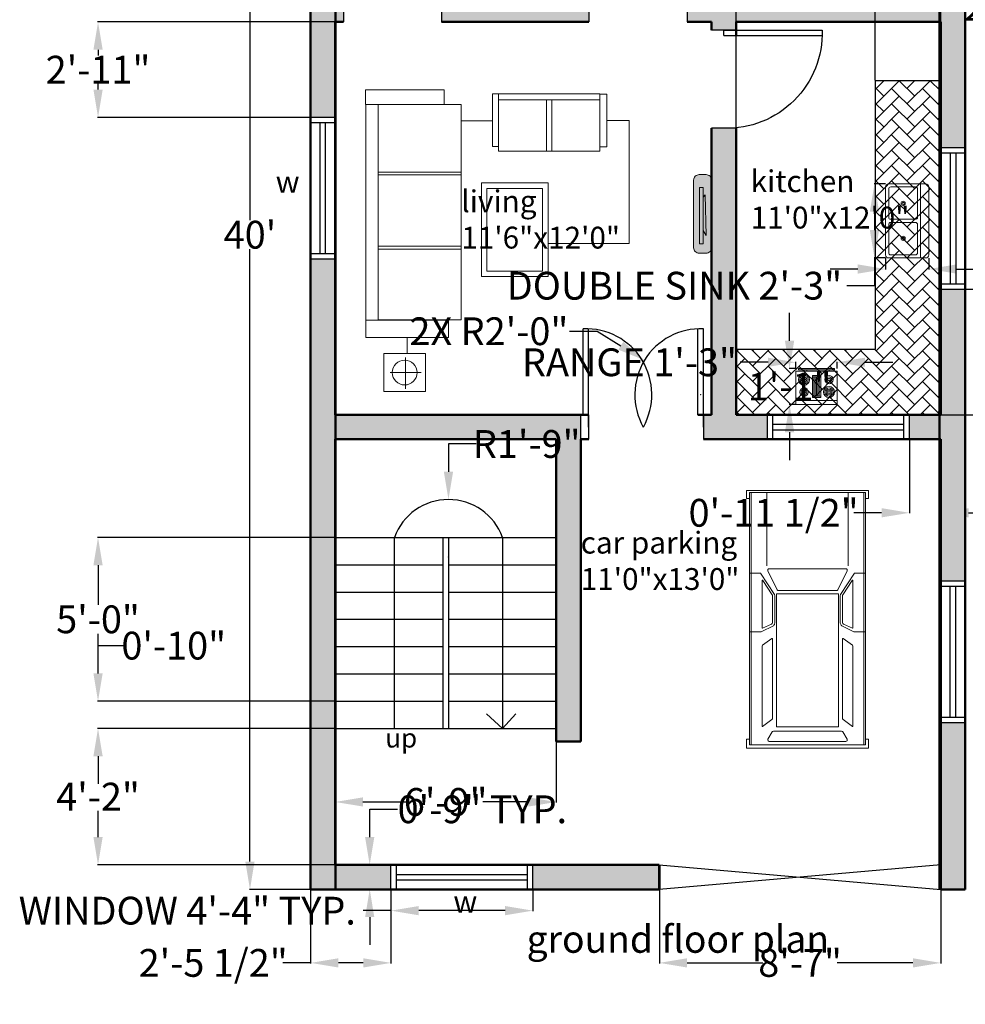
# Model space of a CAD drawing. Units: inches. Extents: x 4451 to 5261, y 886 to 1442.
# Tile 1 of 4: x 4460 to 4807, y 886 to 1247. Entities that reach past the tile are written whole.
import ezdxf

# ---------------------------------------------------------------- set-up
doc = ezdxf.new("R2010")
doc.units = ezdxf.units.IN
doc.header["$MEASUREMENT"] = 0
for name, color, linetype, lineweight in [('A-ANNO-DIMS', 2, 'Continuous', 18), ('A-ANNO-TEXT', 7, 'Continuous', 25), ('A-AREA-IDEN', 7, 'Continuous', 25), ('A-CASE', 9, 'Continuous', 25), ('A-DOOR', 4, 'Continuous', 25), ('A-FLOR-FIXT', 9, 'Continuous', 20), ('A-FLOR-STRS', 7, 'Continuous', 25), ('A-FURN', 8, 'Continuous', 18), ('A-FURN-PATT', 8, 'Continuous', 13), ('A-GLAZ', 4, 'Continuous', 25), ('A-SITE-VEHI', 8, 'Continuous', 13), ('A-WALL', 7, 'Continuous', 50), ('A-WALL-PATT', 252, 'Continuous', 13)]:
    doc.layers.add(name, color=color, linetype=linetype, lineweight=lineweight)
doc.layers.add('A-CASE-PATT', color=11, linetype='Continuous', lineweight=13, true_color=0xf27172)
doc.layers.add('A-EQPM', color=241, linetype='Continuous', lineweight=18, true_color=0xf7abae)
doc.styles.get("Standard").update_dxf_attribs({"font": 'arial.ttf'})
doc.dimstyles.get("Standard").update_dxf_attribs({"dimtxt": 10.18, "dimasz": 10.18, "dimexe": 0.18, "dimexo": 0.0625, "dimgap": 0.09, "dimtad": 0, "dimtih": 1, "dimtoh": 1, "dimdec": 0, "dimzin": 0, "dimdsep": 46, "dimlunit": 3, "dimtxsty": 'Standard', "dimcen": 0.09, "dimadec": 0, "dimazin": 0, "dimtfac": 1, "dimtdec": 0, "dimtofl": 0, "dimtmove": 0, "dimatfit": 3, "dimfxl": 1, "dimtolj": 1, "dimtzin": 0, "dimarcsym": 0})

# ---------------------------------------------------------------- blocks, each defined once
blk = doc.blocks.new('*U5')
for p, q in [((1.28, 38.87), (175.66, 38.87)), ((1.28, 28.15), (52.13, 28.15)), ((1.28, -28.15), (52.13, -28.15)), ((1.28, -38.87), (175.66, -38.87))]:
    blk.add_line(p, q)
for points in [[(5.57, 40.01), (5.57, 42.18), (0, 42.18), (0, -42.18), (5.57, -42.18), (5.57, -40.01), (1.28, -40.01), (1.28, 40.01)], [(171.74, 40.01), (175.66, 40.01), (175.66, -40.01), (171.74, -40.01), (171.74, -42.18), (178.14, -42.18), (178.14, 42.18), (171.74, 42.18)], [(1.28, 40.01), (175.66, 40.01), (175.66, -40.01), (1.28, -40.01)], [(71.47, 21.48), (163.42, 21.48), (163.42, -21.48), (71.47, -21.48)]]:
    blk.add_lwpolyline(points, close=True)
for points in [[(57.15, 40.01), (57.15, 32.39), (71.72, 22.83, 0.086577), (72.56, 22.68), (91.59, 22.68, 0.227875), (93.54, 23.62), (97.72, 32.11), (97.72, 40.01)], [(57.15, -40.01), (57.15, -32.39), (71.72, -22.83, -0.086577), (72.56, -22.68), (91.59, -22.68, -0.227875), (93.54, -23.62), (97.72, -32.11), (97.72, -40.01)]]:
    blk.add_lwpolyline(points, format="xyb")
for points in [[(55.49, 27.42), (68.59, 20.89, -0.284287), (69.14, 19.99), (69.14, -19.99, -0.284287), (68.59, -20.89), (55.49, -27.42, -0.557284), (54.05, -26.53), (54.05, 26.53, -0.557284)], [(62.08, 30.95), (72.14, 24.35, 0.146139), (72.69, 24.18), (91.42, 24.18, 0.29766), (92.33, 24.78), (95.09, 31.05, 0.541236), (94.86, 31.41), (62.21, 31.41, 0.744989)], [(102.19, 24.58), (106.97, 31, -0.236929), (107.78, 31.41), (162.91, 31.41, -0.621576), (163.11, 31), (158.19, 24.58, -0.233368), (157.39, 24.18), (102.39, 24.18, -0.616908)], [(171.88, 27.31), (166.83, 24.47, 0.271143), (166.32, 23.6), (166.32, -23.6, 0.271143), (166.83, -24.47), (171.88, -27.31, 0.573387), (173.37, -26.44), (173.37, 26.44, 0.573387)], [(62.08, -30.95), (72.14, -24.35, -0.146139), (72.69, -24.18), (91.42, -24.18, -0.29766), (92.33, -24.78), (95.09, -31.05, -0.541236), (94.86, -31.41), (62.21, -31.41, -0.744989)], [(102.19, -24.58), (106.97, -31, 0.236929), (107.78, -31.41), (162.91, -31.41, 0.621576), (163.11, -31), (158.19, -24.58, 0.233368), (157.39, -24.18), (102.39, -24.18, 0.616908)]]:
    blk.add_lwpolyline(points, format="xyb", close=True)
blk = doc.blocks.new('Range-Oven - 30 in top')
for p, q in [((0, -3), (30, -3)), ((12, -6), (18, -6)), ((13, -20), (13, -6)), ((14, -6), (14, -20)), ((15, -20), (15, -6)), ((16, -6), (16, -20)), ((17, -20), (17, -6)), ((18, -20), (12, -20)), ((6, -24), (6, -25)), ((8, -25), (8, -24)), ((22, -25), (22, -24)), ((24, -24), (24, -25))]:
    blk.add_line(p, q)
for points in [[(0, -24), (0, 0), (30, 0), (30, -24)], [(12, -21), (12, -5), (18, -5), (18, -21)], [(2, -26), (2, -25), (28, -25), (28, -26)]]:
    blk.add_lwpolyline(points, close=True)
for centre, radius in [((6, -9), 4), ((6, -9), 3), ((6, -9), 2), ((24, -9), 3), ((24, -9), 2), ((6, -9), 1), ((24, -18), 4), ((24, -9), 1), ((6, -18), 3), ((6, -18), 2), ((6, -18), 1), ((24, -18), 3), ((24, -18), 2), ((24, -18), 1)]:
    blk.add_circle(centre, radius)
blk = doc.blocks.new('Sink-double - 36 in top')
for p, q in [((-18, -4), (18, -4)), ((-0.75, -18.5), (-0.75, -6.5)), ((0.75, -6.5), (0.75, -18.5))]:
    blk.add_line(p, q)
for points in [[(-16.5, 0), (16.5, 0)], [(-18, -19.5), (-18, -1.5)], [(18, -1.5), (18, -19.5)], [(-16.5, -18.5), (-16.5, -6.5)], [(-15.5, -5.5), (-1.75, -5.5)], [(1.75, -5.5), (15.5, -5.5)], [(16.5, -6.5), (16.5, -18.5)], [(16.5, -21), (-16.5, -21)], [(-1.75, -19.5), (-15.5, -19.5)], [(15.5, -19.5), (1.75, -19.5)]]:
    blk.add_lwpolyline(points)
for centre, radius in [((-8.5, -12.5), 1), ((-8.5, -12.5), 0.5), ((8.5, -12.5), 1), ((8.5, -12.5), 0.5)]:
    blk.add_circle(centre, radius)
for centre, radius, start, end in [((-16.5, -1.5), 1.5, 90, 180), ((16.5, -1.5), 1.5, 0, 90), ((-15.5, -6.5), 1, 90, 180), ((-1.75, -6.5), 1, 0, 90), ((1.75, -6.5), 1, 90, 180), ((15.5, -6.5), 1, 0, 90), ((-15.5, -18.5), 1, 180, 270), ((-1.75, -18.5), 1, 270, 0), ((1.75, -18.5), 1, 180, 270), ((15.5, -18.5), 1, 270, 0), ((-16.5, -19.5), 1.5, 180, 270), ((16.5, -19.5), 1.5, 270, 0)]:
    blk.add_arc(centre, radius, start, end)
blk = doc.blocks.new('*D12')
at = {"layer": 'A-ANNO-DIMS', "color": 0, "lineweight": -2, "transparency": 16777216}
for p, q in [((4567.03, 1408.25), (4544.66, 1408.25)), ((4544.84, 1398.07), (4544.84, 1173.54)), ((4544.84, 938.43), (4544.84, 1162.96)), ((4567.03, 928.25), (4544.66, 928.25))]:
    blk.add_line(p, q, dxfattribs=at)
at = {"layer": 'A-ANNO-DIMS', "color": 0, "transparency": 16777216}
for points in [[(4543.14, 1398.07), (4546.53, 1398.07), (4544.84, 1408.25)], [(4543.14, 938.43), (4546.53, 938.43), (4544.84, 928.25)]]:
    blk.add_solid(points, dxfattribs=at)
at = {"layer": 'Defpoints', "color": 0, "transparency": 16777216}
for p in [(4567.09, 1408.25), (4544.84, 928.25), (4567.09, 928.25)]:
    blk.add_point(p, dxfattribs=at)
at = {"layer": 'A-ANNO-DIMS', "color": 0, "transparency": 16777216, "insert": (4544.84, 1168.25), "char_height": 10.18, "attachment_point": 5}
blk.add_mtext("\\A1;40'", dxfattribs=at)
blk = doc.blocks.new('DOOR-36-SWING')
for p, q in [((36.01, 36.01), (0.01, 36.01)), ((36.01, 34.01), (0.01, 34.01)), ((31.51, 36.01), (40.51, 36.01)), ((36.01, 34.01), (36.01, 36.01)), ((31.51, 0.01), (40.51, 0.01))]:
    blk.add_line(p, q)
blk.add_arc((35.01, 35.01), 35.01, 178.3634, 271.6366)
blk = doc.blocks.new('WIN-48-PLAN')
for p, q in [((0, 52), (9, 52)), ((0, 50), (9, 50)), ((3.5, 50), (3.5, 2)), ((5.5, 50), (5.5, 2)), ((0, 2), (9, 2)), ((0, 0), (9, 0))]:
    blk.add_line(p, q)
blk = doc.blocks.new('*D21')
at = {"layer": 'A-ANNO-DIMS', "color": 0, "lineweight": -2, "transparency": 16777216}
for p, q in [((4596.54, 928.19), (4596.54, 920.27)), ((4648.54, 928.19), (4648.54, 920.27)), ((4596.54, 920.45), (4586.36, 920.45)), ((4638.36, 920.45), (4606.72, 920.45))]:
    blk.add_line(p, q, dxfattribs=at)
at = {"layer": 'A-ANNO-DIMS', "color": 0, "transparency": 16777216}
for points in [[(4606.72, 922.15), (4606.72, 918.76), (4596.54, 920.45)], [(4638.36, 922.15), (4638.36, 918.76), (4648.54, 920.45)]]:
    blk.add_solid(points, dxfattribs=at)
at = {"layer": 'Defpoints', "color": 0, "transparency": 16777216}
for p in [(4596.54, 928.25), (4648.54, 928.25), (4596.54, 920.45)]:
    blk.add_point(p, dxfattribs=at)
at = {"layer": 'A-ANNO-DIMS', "color": 0, "transparency": 16777216, "insert": (4521.86, 920.45), "char_height": 10.18, "attachment_point": 5}
blk.add_mtext('\\A1;WINDOW 4\'-4" TYP.', dxfattribs=at)
blk = doc.blocks.new('*D22')
at = {"layer": 'A-ANNO-DIMS', "color": 0, "lineweight": -2, "transparency": 16777216}
for p, q in [((4588.74, 947.43), (4588.74, 957.61)), ((4588.74, 957.61), (4598.92, 957.61)), ((4596.47, 937.25), (4588.56, 937.25)), ((4596.47, 928.25), (4588.56, 928.25)), ((4588.74, 918.07), (4588.74, 907.89))]:
    blk.add_line(p, q, dxfattribs=at)
at = {"layer": 'A-ANNO-DIMS', "color": 0, "transparency": 16777216}
for points in [[(4587.04, 947.43), (4590.43, 947.43), (4588.74, 937.25)], [(4587.04, 918.07), (4590.43, 918.07), (4588.74, 928.25)]]:
    blk.add_solid(points, dxfattribs=at)
at = {"layer": 'Defpoints', "color": 0, "transparency": 16777216}
for p in [(4588.74, 937.25), (4596.54, 937.25), (4596.54, 928.25)]:
    blk.add_point(p, dxfattribs=at)
at = {"layer": 'A-ANNO-DIMS', "color": 0, "transparency": 16777216, "insert": (4630.03, 957.61), "char_height": 10.18, "attachment_point": 5}
blk.add_mtext('\\A1;0\'-9" TYP.', dxfattribs=at)
blk = doc.blocks.new('*D27')
at = {"layer": 'A-ANNO-DIMS', "color": 0, "lineweight": -2, "transparency": 16777216}
for p, q in [((4734.76, 1121.48), (4724.58, 1121.48)), ((4744.94, 1119.26), (4744.94, 1121.66)), ((4760.17, 1119.26), (4760.17, 1121.66)), ((4770.35, 1121.48), (4780.53, 1121.48))]:
    blk.add_line(p, q, dxfattribs=at)
at = {"layer": 'A-ANNO-DIMS', "color": 0, "transparency": 16777216}
for points in [[(4734.76, 1123.18), (4734.76, 1119.79), (4744.94, 1121.48)], [(4770.35, 1123.18), (4770.35, 1119.79), (4760.17, 1121.48)]]:
    blk.add_solid(points, dxfattribs=at)
at = {"layer": 'Defpoints', "color": 0, "transparency": 16777216}
for p in [(4744.94, 1121.48), (4744.94, 1119.2), (4760.17, 1119.2)]:
    blk.add_point(p, dxfattribs=at)
at = {"layer": 'A-ANNO-DIMS', "color": 0, "transparency": 16777216, "insert": (4683.96, 1121.48), "char_height": 10.18, "attachment_point": 5}
blk.add_mtext('\\A1;RANGE 1\'-3"', dxfattribs=at)
blk = doc.blocks.new('*D28')
at = {"layer": 'A-ANNO-DIMS', "color": 0, "lineweight": -2, "transparency": 16777216}
for p, q in [((4742.66, 1129.38), (4742.66, 1139.56)), ((4744.88, 1119.2), (4742.48, 1119.2)), ((4744.88, 1106), (4742.48, 1106)), ((4742.66, 1095.82), (4742.66, 1085.64))]:
    blk.add_line(p, q, dxfattribs=at)
at = {"layer": 'A-ANNO-DIMS', "color": 0, "transparency": 16777216}
for points in [[(4740.96, 1129.38), (4744.36, 1129.38), (4742.66, 1119.2)], [(4740.96, 1095.82), (4744.36, 1095.82), (4742.66, 1106)]]:
    blk.add_solid(points, dxfattribs=at)
at = {"layer": 'Defpoints', "color": 0, "transparency": 16777216}
for p in [(4744.94, 1119.2), (4742.66, 1106), (4744.94, 1106)]:
    blk.add_point(p, dxfattribs=at)
at = {"layer": 'A-ANNO-DIMS', "color": 0, "transparency": 16777216, "insert": (4742.66, 1112.6), "char_height": 10.18, "attachment_point": 5}
blk.add_mtext('\\A1;1\'-1"', dxfattribs=at)
blk = doc.blocks.new('*D29')
at = {"layer": 'A-ANNO-DIMS', "color": 0, "lineweight": -2, "transparency": 16777216}
for p, q in [((4777.81, 1186.9), (4773.62, 1186.9)), ((4773.8, 1176.72), (4773.8, 1169.92)), ((4777.81, 1159.74), (4773.62, 1159.74)), ((4773.8, 1159.74), (4773.8, 1149.56)), ((4773.8, 1149.56), (4763.62, 1149.56))]:
    blk.add_line(p, q, dxfattribs=at)
at = {"layer": 'A-ANNO-DIMS', "color": 0, "transparency": 16777216}
for points in [[(4772.1, 1176.72), (4775.49, 1176.72), (4773.8, 1186.9)], [(4772.1, 1169.92), (4775.49, 1169.92), (4773.8, 1159.74)]]:
    blk.add_solid(points, dxfattribs=at)
at = {"layer": 'Defpoints', "color": 0, "transparency": 16777216}
for p in [(4777.87, 1186.9), (4773.8, 1159.74), (4777.87, 1159.74)]:
    blk.add_point(p, dxfattribs=at)
at = {"layer": 'A-ANNO-DIMS', "color": 0, "transparency": 16777216, "insert": (4700.46, 1149.56), "char_height": 10.18, "attachment_point": 5}
blk.add_mtext('\\A1;DOUBLE SINK 2\'-3"', dxfattribs=at)
blk = doc.blocks.new('*D30')
at = {"layer": 'A-ANNO-DIMS', "color": 0, "lineweight": -2, "transparency": 16777216}
for p, q in [((4777.87, 1159.67), (4777.87, 1155.48)), ((4793.72, 1159.67), (4793.72, 1155.48)), ((4767.69, 1155.66), (4757.51, 1155.66)), ((4803.9, 1155.66), (4814.08, 1155.66))]:
    blk.add_line(p, q, dxfattribs=at)
at = {"layer": 'A-ANNO-DIMS', "color": 0, "transparency": 16777216}
for points in [[(4767.69, 1157.36), (4767.69, 1153.97), (4777.87, 1155.66)], [(4803.9, 1157.36), (4803.9, 1153.97), (4793.72, 1155.66)]]:
    blk.add_solid(points, dxfattribs=at)
at = {"layer": 'Defpoints', "color": 0, "transparency": 16777216}
for p in [(4777.87, 1159.74), (4793.72, 1159.74), (4793.72, 1155.66)]:
    blk.add_point(p, dxfattribs=at)
at = {"layer": 'A-ANNO-DIMS', "color": 0, "transparency": 16777216, "insert": (4827.22, 1155.66), "char_height": 10.18, "attachment_point": 5}
blk.add_mtext('\\A1;1\'-4"', dxfattribs=at)
blk = doc.blocks.new('*D41')
at = {"layer": 'A-ANNO-DIMS', "color": 0, "lineweight": -2, "transparency": 16777216}
for p, q in [((4723.09, 1102.31), (4723.09, 1435.38)), ((4733.27, 1435.2), (4746.94, 1435.2)), ((4787.91, 1435.2), (4774.24, 1435.2)), ((4798.09, 1102.31), (4798.09, 1435.38))]:
    blk.add_line(p, q, dxfattribs=at)
at = {"layer": 'A-ANNO-DIMS', "color": 0, "transparency": 16777216}
for points in [[(4733.27, 1436.9), (4733.27, 1433.51), (4723.09, 1435.2)], [(4787.91, 1436.9), (4787.91, 1433.51), (4798.09, 1435.2)]]:
    blk.add_solid(points, dxfattribs=at)
at = {"layer": 'Defpoints', "color": 0, "transparency": 16777216}
for p in [(4798.09, 1435.2), (4723.09, 1102.25), (4798.09, 1102.25)]:
    blk.add_point(p, dxfattribs=at)
at = {"layer": 'A-ANNO-DIMS', "color": 0, "transparency": 16777216, "insert": (4760.59, 1435.2), "char_height": 10.18, "attachment_point": 5}
blk.add_mtext('\\A1;6\'-3"', dxfattribs=at)
blk = doc.blocks.new('*D42')
at = {"layer": 'A-ANNO-DIMS', "color": 0, "lineweight": -2, "transparency": 16777216}
for p, q in [((4694.94, 928.2), (4694.94, 901.12)), ((4798.09, 928.19), (4798.09, 901.12)), ((4705.12, 901.3), (4732.89, 901.3)), ((4787.91, 901.3), (4760.15, 901.3))]:
    blk.add_line(p, q, dxfattribs=at)
at = {"layer": 'A-ANNO-DIMS', "color": 0, "transparency": 16777216}
for points in [[(4705.12, 903), (4705.12, 899.61), (4694.94, 901.3)], [(4787.91, 903), (4787.91, 899.61), (4798.09, 901.3)]]:
    blk.add_solid(points, dxfattribs=at)
at = {"layer": 'Defpoints', "color": 0, "transparency": 16777216}
for p in [(4694.94, 928.26), (4798.09, 928.25), (4798.09, 901.3)]:
    blk.add_point(p, dxfattribs=at)
at = {"layer": 'A-ANNO-DIMS', "color": 0, "transparency": 16777216, "insert": (4746.52, 901.3), "char_height": 10.18, "attachment_point": 5}
blk.add_mtext('\\A1;8\'-7"', dxfattribs=at)
blk = doc.blocks.new('*D43')
at = {"layer": 'A-ANNO-DIMS', "color": 0, "lineweight": -2, "transparency": 16777216}
for p, q in [((4567.09, 928.19), (4567.09, 901.12)), ((4596.54, 928.19), (4596.54, 901.12)), ((4567.09, 901.3), (4556.91, 901.3)), ((4586.36, 901.3), (4577.27, 901.3))]:
    blk.add_line(p, q, dxfattribs=at)
at = {"layer": 'A-ANNO-DIMS', "color": 0, "transparency": 16777216}
for points in [[(4577.27, 903), (4577.27, 899.61), (4567.09, 901.3)], [(4586.36, 903), (4586.36, 899.61), (4596.54, 901.3)]]:
    blk.add_solid(points, dxfattribs=at)
at = {"layer": 'Defpoints', "color": 0, "transparency": 16777216}
for p in [(4567.09, 928.25), (4596.54, 928.25), (4567.09, 901.3)]:
    blk.add_point(p, dxfattribs=at)
at = {"layer": 'A-ANNO-DIMS', "color": 0, "transparency": 16777216, "insert": (4531.35, 901.3), "char_height": 10.18, "attachment_point": 5}
blk.add_mtext('\\A1;2\'-5 1/2"', dxfattribs=at)
blk = doc.blocks.new('*D45')
at = {"layer": 'A-ANNO-DIMS', "color": 0, "lineweight": -2, "transparency": 16777216}
for p, q in [((4798.16, 1148.25), (4859.61, 1148.25)), ((4859.43, 1138.07), (4859.43, 1130.54)), ((4859.43, 1112.43), (4859.43, 1119.96)), ((4798.16, 1102.25), (4859.61, 1102.25))]:
    blk.add_line(p, q, dxfattribs=at)
at = {"layer": 'A-ANNO-DIMS', "color": 0, "transparency": 16777216}
for points in [[(4857.74, 1138.07), (4861.13, 1138.07), (4859.43, 1148.25)], [(4857.74, 1112.43), (4861.13, 1112.43), (4859.43, 1102.25)]]:
    blk.add_solid(points, dxfattribs=at)
at = {"layer": 'Defpoints', "color": 0, "transparency": 16777216}
for p in [(4798.09, 1148.25), (4859.43, 1148.25), (4798.09, 1102.25)]:
    blk.add_point(p, dxfattribs=at)
at = {"layer": 'A-ANNO-DIMS', "color": 0, "transparency": 16777216, "insert": (4859.43, 1125.25), "char_height": 10.18, "attachment_point": 5}
blk.add_mtext('\\A1;3\'-10"', dxfattribs=at)
blk = doc.blocks.new('*D48')
at = {"layer": 'A-ANNO-DIMS', "color": 0, "lineweight": -2, "transparency": 16777216}
for p, q in [((4576.03, 1246.25), (4488.96, 1246.25)), ((4489.14, 1236.07), (4489.14, 1233.95)), ((4489.14, 1221.44), (4489.14, 1223.55)), ((4576.03, 1211.26), (4488.96, 1211.26))]:
    blk.add_line(p, q, dxfattribs=at)
at = {"layer": 'A-ANNO-DIMS', "color": 0, "transparency": 16777216}
for points in [[(4487.45, 1236.07), (4490.84, 1236.07), (4489.14, 1246.25)], [(4487.45, 1221.44), (4490.84, 1221.44), (4489.14, 1211.26)]]:
    blk.add_solid(points, dxfattribs=at)
at = {"layer": 'Defpoints', "color": 0, "transparency": 16777216}
for p in [(4576.09, 1246.25), (4489.14, 1211.26), (4576.09, 1211.26)]:
    blk.add_point(p, dxfattribs=at)
at = {"layer": 'A-ANNO-DIMS', "color": 0, "transparency": 16777216, "insert": (4489.14, 1228.75), "char_height": 10.18, "attachment_point": 5}
blk.add_mtext('\\A1;2\'-11"', dxfattribs=at)
blk = doc.blocks.new('*D51')
at = {"layer": 'A-ANNO-DIMS', "color": 0, "lineweight": -2, "transparency": 16777216}
for p, q in [((4489.14, 1007.43), (4489.14, 1017.61)), ((4489.14, 1017.61), (4499.32, 1017.61)), ((4576.03, 997.25), (4488.96, 997.25)), ((4576.03, 987.25), (4488.96, 987.25)), ((4489.14, 977.07), (4489.14, 966.89))]:
    blk.add_line(p, q, dxfattribs=at)
at = {"layer": 'A-ANNO-DIMS', "color": 0, "transparency": 16777216}
for points in [[(4487.45, 1007.43), (4490.84, 1007.43), (4489.14, 997.25)], [(4487.45, 977.07), (4490.84, 977.07), (4489.14, 987.25)]]:
    blk.add_solid(points, dxfattribs=at)
at = {"layer": 'Defpoints', "color": 0, "transparency": 16777216}
for p in [(4489.14, 997.25), (4576.09, 997.25), (4576.09, 987.25)]:
    blk.add_point(p, dxfattribs=at)
at = {"layer": 'A-ANNO-DIMS', "color": 0, "transparency": 16777216, "insert": (4516.9, 1017.61), "char_height": 10.18, "attachment_point": 5}
blk.add_mtext('\\A1;0\'-10"', dxfattribs=at)
blk = doc.blocks.new('*D52')
at = {"layer": 'A-ANNO-DIMS', "color": 0, "lineweight": -2, "transparency": 16777216}
for p, q in [((4576.03, 1057.25), (4488.96, 1057.25)), ((4489.14, 1047.07), (4489.14, 1032.54)), ((4489.14, 1007.43), (4489.14, 1021.96)), ((4576.03, 997.25), (4488.96, 997.25))]:
    blk.add_line(p, q, dxfattribs=at)
at = {"layer": 'A-ANNO-DIMS', "color": 0, "transparency": 16777216}
for points in [[(4487.45, 1047.07), (4490.84, 1047.07), (4489.14, 1057.25)], [(4487.45, 1007.43), (4490.84, 1007.43), (4489.14, 997.25)]]:
    blk.add_solid(points, dxfattribs=at)
at = {"layer": 'Defpoints', "color": 0, "transparency": 16777216}
for p in [(4489.14, 1057.25), (4576.09, 1057.25), (4576.09, 997.25)]:
    blk.add_point(p, dxfattribs=at)
at = {"layer": 'A-ANNO-DIMS', "color": 0, "transparency": 16777216, "insert": (4489.14, 1027.25), "char_height": 10.18, "attachment_point": 5}
blk.add_mtext('\\A1;5\'-0"', dxfattribs=at)
blk = doc.blocks.new('*D53')
at = {"layer": 'A-ANNO-DIMS', "color": 0, "lineweight": -2, "transparency": 16777216}
for p, q in [((4576.03, 987.25), (4488.96, 987.25)), ((4489.14, 977.07), (4489.14, 967.45)), ((4489.14, 947.43), (4489.14, 957.05)), ((4576.03, 937.25), (4488.96, 937.25))]:
    blk.add_line(p, q, dxfattribs=at)
at = {"layer": 'A-ANNO-DIMS', "color": 0, "transparency": 16777216}
for points in [[(4487.45, 977.07), (4490.84, 977.07), (4489.14, 987.25)], [(4487.45, 947.43), (4490.84, 947.43), (4489.14, 937.25)]]:
    blk.add_solid(points, dxfattribs=at)
at = {"layer": 'Defpoints', "color": 0, "transparency": 16777216}
for p in [(4489.14, 987.25), (4576.09, 987.25), (4576.09, 937.25)]:
    blk.add_point(p, dxfattribs=at)
at = {"layer": 'A-ANNO-DIMS', "color": 0, "transparency": 16777216, "insert": (4489.14, 962.25), "char_height": 10.18, "attachment_point": 5}
blk.add_mtext('\\A1;4\'-2"', dxfattribs=at)
blk = doc.blocks.new('*D54')
at = {"layer": 'A-ANNO-DIMS', "color": 0, "lineweight": -2, "transparency": 16777216}
for p, q in [((4774.09, 1224.89), (4774.09, 1251.96)), ((4784.27, 1251.78), (4787.91, 1251.78)), ((4798.09, 1224.89), (4798.09, 1251.96)), ((4798.09, 1251.78), (4808.27, 1251.78))]:
    blk.add_line(p, q, dxfattribs=at)
at = {"layer": 'A-ANNO-DIMS', "color": 0, "transparency": 16777216}
for points in [[(4784.27, 1253.48), (4784.27, 1250.08), (4774.09, 1251.78)], [(4787.91, 1253.48), (4787.91, 1250.08), (4798.09, 1251.78)]]:
    blk.add_solid(points, dxfattribs=at)
at = {"layer": 'Defpoints', "color": 0, "transparency": 16777216}
for p in [(4798.09, 1251.78), (4774.09, 1224.83), (4798.09, 1224.83)]:
    blk.add_point(p, dxfattribs=at)
at = {"layer": 'A-ANNO-DIMS', "color": 0, "transparency": 16777216, "insert": (4821.98, 1251.78), "char_height": 10.18, "attachment_point": 5}
blk.add_mtext('\\A1;2\'-0"', dxfattribs=at)
blk = doc.blocks.new('*D55')
at = {"layer": 'A-ANNO-DIMS', "color": 0, "lineweight": -2, "transparency": 16777216}
for p, q in [((4786.59, 1093.19), (4786.59, 1066.12)), ((4798.09, 1093.19), (4798.09, 1066.12)), ((4776.41, 1066.3), (4766.23, 1066.3)), ((4808.27, 1066.3), (4818.45, 1066.3))]:
    blk.add_line(p, q, dxfattribs=at)
at = {"layer": 'A-ANNO-DIMS', "color": 0, "transparency": 16777216}
for points in [[(4776.41, 1068), (4776.41, 1064.61), (4786.59, 1066.3)], [(4808.27, 1068), (4808.27, 1064.61), (4798.09, 1066.3)]]:
    blk.add_solid(points, dxfattribs=at)
at = {"layer": 'Defpoints', "color": 0, "transparency": 16777216}
for p in [(4786.59, 1093.25), (4798.09, 1093.25), (4786.59, 1066.3)]:
    blk.add_point(p, dxfattribs=at)
at = {"layer": 'A-ANNO-DIMS', "color": 0, "transparency": 16777216, "insert": (4736.8, 1066.3), "char_height": 10.18, "attachment_point": 5}
blk.add_mtext('\\A1;0\'-11 1/2"', dxfattribs=at)
blk = doc.blocks.new('*D56')
at = {"layer": 'A-ANNO-DIMS', "color": 0, "lineweight": -2, "transparency": 16777216}
for p, q in [((4576.09, 987.19), (4576.09, 960.12)), ((4657.09, 987.19), (4657.09, 960.12)), ((4586.27, 960.3), (4602.94, 960.3)), ((4646.91, 960.3), (4630.24, 960.3))]:
    blk.add_line(p, q, dxfattribs=at)
at = {"layer": 'A-ANNO-DIMS', "color": 0, "transparency": 16777216}
for points in [[(4586.27, 962), (4586.27, 958.61), (4576.09, 960.3)], [(4646.91, 962), (4646.91, 958.61), (4657.09, 960.3)]]:
    blk.add_solid(points, dxfattribs=at)
at = {"layer": 'Defpoints', "color": 0, "transparency": 16777216}
for p in [(4576.09, 987.25), (4657.09, 987.25), (4576.09, 960.3)]:
    blk.add_point(p, dxfattribs=at)
at = {"layer": 'A-ANNO-DIMS', "color": 0, "transparency": 16777216, "insert": (4616.59, 960.3), "char_height": 10.18, "attachment_point": 5}
blk.add_mtext('\\A1;6\'-9"', dxfattribs=at)
blk = doc.blocks.new('*D82')
at = {"layer": 'A-ANNO-DIMS', "color": 0, "lineweight": -2, "transparency": 16777216}
for p, q in [((4661.95, 1132.86), (4672.13, 1132.86)), ((4672.13, 1132.86), (4680.81, 1127.55)), ((4710, 1109.62), (4710.18, 1109.62)), ((4710.09, 1109.53), (4710.09, 1109.71))]:
    blk.add_line(p, q, dxfattribs=at)
at = {"layer": 'A-ANNO-DIMS', "color": 0, "transparency": 16777216}
blk.add_solid([(4681.7, 1128.99), (4679.92, 1126.1), (4689.49, 1122.23)], dxfattribs=at)
at = {"layer": 'Defpoints', "color": 0, "transparency": 16777216}
for p in [(4689.49, 1122.23), (4710.09, 1109.62)]:
    blk.add_point(p, dxfattribs=at)
at = {"layer": 'A-ANNO-DIMS', "color": 0, "transparency": 16777216, "insert": (4632.43, 1132.86), "char_height": 10.18, "attachment_point": 5}
blk.add_mtext('\\A1;2X R2\'-0"', dxfattribs=at)
blk = doc.blocks.new('*D83')
at = {"layer": 'A-ANNO-DIMS', "color": 0, "lineweight": -2, "transparency": 16777216}
for p, q in [((4627.79, 1091.53), (4617.61, 1091.53)), ((4617.61, 1091.53), (4617.61, 1081.35)), ((4617.52, 1050.09), (4617.7, 1050.09)), ((4617.61, 1050), (4617.61, 1050.18))]:
    blk.add_line(p, q, dxfattribs=at)
at = {"layer": 'A-ANNO-DIMS', "color": 0, "transparency": 16777216}
blk.add_solid([(4615.92, 1081.35), (4619.31, 1081.35), (4617.61, 1071.17)], dxfattribs=at)
at = {"layer": 'Defpoints', "color": 0, "transparency": 16777216}
for p in [(4617.61, 1071.17), (4617.61, 1050.09)]:
    blk.add_point(p, dxfattribs=at)
at = {"layer": 'A-ANNO-DIMS', "color": 0, "transparency": 16777216, "insert": (4646.29, 1091.53), "char_height": 10.18, "attachment_point": 5}
blk.add_mtext('\\A1;R1\'-9"', dxfattribs=at)

msp = doc.modelspace()

# ---------------------------------------------------------------- hatches: boundary and pattern name
at = {"layer": 'A-CASE-PATT'}
h = msp.add_hatch(dxfattribs=at)
h.set_pattern_fill('AR-HBONE', color=256)
h.paths.add_polyline_path([(4798.09, 1224.83), (4774.09, 1224.83), (4774.09, 1126.25), (4723.09, 1126.25), (4723.09, 1102.25), (4798.09, 1102.25)])
at = {"layer": 'A-FURN-PATT'}
h = msp.add_hatch(color=256, dxfattribs=at)
h.dxf.hatch_style = 1
h.paths.add_polyline_path([(4714.09, 1188.28, 0.414214), (4712.09, 1190.28), (4709.5, 1190.28, 0.414214), (4707.5, 1188.28), (4707.5, 1163.46, 0.414214), (4709.5, 1161.46), (4712.09, 1161.46, 0.414214), (4714.09, 1163.46)])
h.paths.add_polyline_path([(4709.63, 1185.53), (4710.96, 1185.53), (4710.96, 1182.02), (4711.77, 1182.89), (4712.12, 1167.9), (4710.96, 1169.8), (4710.96, 1164.86), (4709.63, 1164.86)], flags=16)
h = msp.add_hatch(color=256, dxfattribs=at)
h.dxf.hatch_style = 1
h.paths.add_polyline_path([(4710.96, 1185.53), (4709.63, 1185.53), (4709.63, 1164.86), (4710.96, 1164.86)])
h.paths.add_polyline_path([(4711.77, 1182.89), (4710.96, 1182.02), (4710.96, 1169.8), (4712.12, 1167.9)])
at = {"layer": 'A-WALL-PATT'}
h = msp.add_hatch(color=256, dxfattribs=at)
h.dxf.hatch_style = 1
h.paths.add_polyline_path([(4706.09, 1408.25), (4567.09, 1408.25), (4567.09, 1386.25), (4576.09, 1386.25), (4576.09, 1399.25), (4657.09, 1399.25), (4657.09, 1396.25), (4661.59, 1396.25), (4666.09, 1396.25), (4666.09, 1399.25), (4706.09, 1399.25)])
h.paths.add_polyline_path([(4807.09, 1408.25), (4758.09, 1408.25), (4758.09, 1399.25), (4798.09, 1399.25), (4798.09, 1353.25), (4807.09, 1353.25)])
h.paths.add_polyline_path([(4807.09, 1301.25), (4798.09, 1301.25), (4798.09, 1292.89), (4798.09, 1255.25), (4705.09, 1255.25), (4705.09, 1252.75, -0.014283), (4705.09, 1250.75), (4705.09, 1246.25), (4714.09, 1246.25), (4714.09, 1243.25), (4723.09, 1243.25), (4723.09, 1246.25), (4798.09, 1246.25), (4798.09, 1200.25), (4807.09, 1200.25)])
h.paths.add_polyline_path([(4666.09, 1360.25), (4661.59, 1360.25, -0.014283), (4659.59, 1360.25), (4657.09, 1360.25), (4657.09, 1345.25), (4576.09, 1345.25), (4576.09, 1358.25), (4567.09, 1358.25), (4567.09, 1309.75), (4576.09, 1309.75), (4576.09, 1336.25), (4657.09, 1336.25), (4657.09, 1255.25), (4615.09, 1255.25), (4615.09, 1252.75, -0.014283), (4615.09, 1250.75), (4615.09, 1246.25), (4669.09, 1246.25), (4669.09, 1255.25), (4666.09, 1255.25)])
h.paths.add_polyline_path([(4576.09, 1281.75), (4567.09, 1281.75), (4567.09, 1211.26), (4576.09, 1211.26), (4576.09, 1246.25), (4579.09, 1246.25), (4579.09, 1255.25), (4576.09, 1255.25)])
h.paths.add_polyline_path([(4666.09, 1102.25), (4576.09, 1102.25), (4576.09, 1159.26), (4567.09, 1159.26), (4567.09, 928.25), (4596.54, 928.25), (4596.54, 937.25), (4576.09, 937.25), (4576.09, 1093.25), (4579.09, 1093.25), (4657.09, 1093.25), (4657.09, 982.46), (4666.09, 982.46), (4666.09, 1093.25)])
h.paths.add_polyline_path([(4723.09, 1207.25), (4720.59, 1207.25, -0.014283), (4718.59, 1207.25), (4714.09, 1207.25), (4714.09, 1102.25), (4711.09, 1102.25), (4711.09, 1097.75), (4711.09, 1093.25), (4734.59, 1093.25), (4734.59, 1102.25), (4723.09, 1102.25)])
h.paths.add_polyline_path([(4807.09, 1148.25), (4798.09, 1148.25), (4798.09, 1102.25), (4786.59, 1102.25), (4786.59, 1093.25), (4798.09, 1093.25), (4798.09, 1041.25), (4807.09, 1041.25)])
h.paths.add_polyline_path([(4694.85, 937.25), (4649.53, 937.25), (4648.54, 937.25), (4648.54, 928.25), (4649.53, 928.25), (4694.85, 928.25)])
h.paths.add_polyline_path([(4807.09, 989.25), (4798.09, 989.25), (4798.09, 937.25), (4798.09, 928.25), (4807.09, 928.25)])
h.paths.add_polyline_path([(4662.88, 1033.63), (4722.94, 1033.63), (4722.94, 1063.48), (4662.88, 1063.48)], flags=9)

# ---------------------------------------------------------------- linework, layer by layer
at = {"layer": 'A-CASE'}
for p, q in [((4774.09, 1224.83), (4774.09, 1126.25)), ((4774.09, 1224.83), (4798.09, 1224.83)), ((4723.09, 1126.25), (4774.09, 1126.25))]:
    msp.add_line(p, q, dxfattribs=at)
at = {"layer": 'A-DOOR'}
for p, q in [((4667.01, 1102.25), (4667.01, 1133.75)), ((4669.01, 1097.75), (4669.01, 1133.75)), ((4709.09, 1102.25), (4709.09, 1133.75)), ((4711.09, 1097.75), (4711.09, 1133.75)), ((4666.09, 1093.25), (4666.09, 1102.25)), ((4669.09, 1093.25), (4669.09, 1102.25)), ((4711.09, 1102.25), (4711.09, 1093.25)), ((4694.85, 937.25), (4798.09, 928.25)), ((4798.09, 937.25), (4694.85, 928.25))]:
    msp.add_line(p, q, dxfattribs=at)
for centre, start, end in [((4668.01, 1109.62), 330.5887, 92.3724), ((4710.09, 1109.62), 87.6276, 209.4113)]:
    msp.add_arc(centre, 24.16, start, end, dxfattribs=at)
at = {"layer": 'A-FLOR-STRS'}
for p, q in [((4576.09, 1093.25), (4576.09, 1057.25)), ((4576.09, 1057.25), (4657.09, 1057.25)), ((4597.78, 987.25), (4597.78, 1057.25)), ((4615.59, 1057.25), (4615.59, 987.25)), ((4617.59, 1057.25), (4617.59, 987.25)), ((4637.44, 1057.25), (4637.44, 987.25)), ((4576.09, 1047.25), (4615.59, 1047.25)), ((4617.59, 1047.25), (4657.09, 1047.25)), ((4576.09, 1037.25), (4615.59, 1037.25)), ((4617.59, 1037.25), (4657.09, 1037.25)), ((4576.09, 1027.25), (4615.59, 1027.25)), ((4617.59, 1027.25), (4657.09, 1027.25)), ((4576.09, 1017.25), (4615.59, 1017.25)), ((4617.59, 1017.25), (4657.09, 1017.25)), ((4576.09, 1007.25), (4615.59, 1007.25)), ((4617.59, 1007.25), (4657.09, 1007.25)), ((4576.09, 997.25), (4615.59, 997.25)), ((4617.59, 997.25), (4657.09, 997.25)), ((4637.44, 987.25), (4631.55, 992.61)), ((4637.44, 987.25), (4642.31, 992.61)), ((4576.09, 987.25), (4657.09, 987.25))]:
    msp.add_line(p, q, dxfattribs=at)
msp.add_arc((4617.61, 1050.09), 21.08, 19.86, 160.14, dxfattribs=at)
at = {"layer": 'A-FURN'}
for p, q in [((4653.52, 1217.67), (4653.52, 1198.84)), ((4655.52, 1217.67), (4655.52, 1198.84)), ((4622.31, 1209.94), (4633.78, 1209.94)), ((4675.72, 1210.1), (4683.87, 1210.1)), ((4683.87, 1210.1), (4683.87, 1165.05)), ((4591.86, 1191.19), (4622.31, 1191.19)), ((4591.86, 1190.19), (4622.31, 1190.19)), ((4710.96, 1182.02), (4711.77, 1182.89)), ((4711.77, 1182.89), (4712.12, 1167.9)), ((4712.12, 1167.9), (4710.96, 1169.8)), ((4591.86, 1164.01), (4622.31, 1164.01)), ((4591.86, 1163.01), (4622.31, 1163.01)), ((4683.87, 1165.05), (4654.13, 1165.05)), ((4602.45, 1130.55), (4602.45, 1124.71)), ((4601.89, 1123.19), (4601.89, 1111.74)), ((4601.55, 1117.71), (4596.19, 1117.71)), ((4596.19, 1117.71), (4607.6, 1117.71))]:
    msp.add_line(p, q, dxfattribs=at)
for points in [[(4616.04, 1215.94), (4616.04, 1215.94), (4587.23, 1215.94), (4587.23, 1215.94), (4587.23, 1221.42), (4587.23, 1221.42), (4616.04, 1221.42), (4616.04, 1221.42)], [(4635.95, 1219.87), (4635.95, 1219.87), (4633.78, 1219.87), (4633.78, 1219.87), (4633.78, 1200.54), (4633.78, 1200.54), (4635.95, 1200.54), (4635.95, 1200.54)], [(4635.95, 1219.87), (4635.95, 1219.87), (4673.1, 1219.87), (4673.1, 1219.87), (4673.1, 1217.67), (4673.1, 1217.67), (4635.95, 1217.67), (4635.95, 1217.67)], [(4635.95, 1217.67), (4635.95, 1217.67), (4673.1, 1217.67), (4673.1, 1217.67), (4673.1, 1198.84), (4673.1, 1198.84), (4635.95, 1198.84), (4635.95, 1198.84)], [(4673.1, 1219.73), (4673.1, 1219.73), (4675.72, 1219.73), (4675.72, 1219.73), (4675.72, 1200.48), (4675.72, 1200.48), (4673.1, 1200.48), (4673.1, 1200.48)], [(4591.86, 1215.94), (4591.86, 1215.94), (4587.32, 1215.94), (4587.32, 1215.94), (4587.32, 1136.87), (4587.32, 1136.87), (4591.86, 1136.87), (4591.86, 1136.87)], [(4622.31, 1215.94), (4622.31, 1215.94), (4591.86, 1215.94), (4591.86, 1215.94), (4591.86, 1137.07), (4591.86, 1137.07), (4622.31, 1137.07), (4622.31, 1137.07)], [(4654.13, 1187.21), (4629.72, 1187.21), (4629.72, 1152.91), (4654.13, 1152.91)], [(4652.13, 1185.21), (4652.13, 1185.21), (4631.72, 1185.21), (4631.72, 1185.21), (4631.72, 1154.91), (4631.72, 1154.91), (4652.13, 1154.91), (4652.13, 1154.91)], [(4710.96, 1185.53), (4710.96, 1185.53), (4709.63, 1185.53), (4709.63, 1185.53), (4709.63, 1164.86), (4709.63, 1164.86), (4710.96, 1164.86), (4710.96, 1164.86)], [(4587.32, 1136.87), (4587.32, 1136.87), (4617.57, 1136.87), (4617.57, 1136.87), (4617.57, 1130.55), (4617.57, 1130.55), (4587.32, 1130.55), (4587.32, 1130.55)], [(4593.94, 1124.71), (4593.94, 1124.71), (4609.17, 1124.71), (4609.17, 1124.71), (4609.17, 1110.72), (4609.17, 1110.72), (4593.94, 1110.72), (4593.94, 1110.72)]]:
    msp.add_lwpolyline(points, close=True, dxfattribs=at)
msp.add_lwpolyline([(4714.09, 1188.28, 0.414214), (4712.09, 1190.28), (4709.5, 1190.28, 0.414214), (4707.5, 1188.28), (4707.5, 1163.46, 0.414214), (4709.5, 1161.46), (4712.09, 1161.46, 0.414214), (4714.09, 1163.46)], format="xyb", close=True, dxfattribs=at)
msp.add_circle((4601.55, 1117.71), 4.53, dxfattribs=at)
at = {"layer": 'A-GLAZ'}
msp.add_line((4803.59, 1198.25), (4803.59, 1150.25), dxfattribs=at)
at = {"layer": 'A-WALL'}
for p, q in [((4567.09, 928.25), (4567.09, 1408.25)), ((4576.2, 928.25), (4576.2, 1408.25)), ((4797.65, 928.29), (4797.65, 1408.25)), ((4807.09, 1408.25), (4807.09, 928.25)), ((4576.09, 1246.25), (4579.09, 1246.25)), ((4576.09, 1102.25), (4576.09, 1246.25)), ((4615.09, 1246.25), (4669.09, 1246.25)), ((4705.09, 1246.25), (4714.09, 1246.25)), ((4714.09, 1243.25), (4714.09, 1246.25)), ((4723.09, 1246.25), (4798.09, 1246.25)), ((4723.09, 1241.25), (4723.09, 1246.25)), ((4798.09, 1246.25), (4798.09, 1102.25)), ((4714.09, 1102.25), (4714.09, 1207.25)), ((4723.09, 1102.25), (4723.09, 1207.41)), ((4576.09, 1102.25), (4669.09, 1102.25)), ((4709.09, 1102.25), (4714.09, 1102.25)), ((4723.09, 1102.25), (4798.09, 1102.25)), ((4576.09, 937.25), (4576.09, 1093.25)), ((4576.09, 1093.25), (4579.09, 1093.25)), ((4579.09, 1093.25), (4657.09, 1093.25)), ((4657.09, 1093.25), (4657.09, 982.46)), ((4666.09, 1093.25), (4666.09, 982.46)), ((4666.09, 1093.25), (4669.09, 1093.25)), ((4711.09, 1093.25), (4798.09, 1093.25)), ((4798.09, 1093.25), (4798.09, 937.25)), ((4657.09, 982.46), (4666.09, 982.46)), ((4649.53, 937.25), (4576.09, 937.25)), ((4694.85, 937.25), (4649.53, 937.25)), ((4694.85, 937.25), (4694.85, 928.25)), ((4694.94, 928.26), (4694.94, 937.24)), ((4798.09, 937.25), (4798.09, 928.25)), ((4649.53, 928.25), (4567.09, 928.25)), ((4694.85, 928.25), (4649.53, 928.25)), ((4807.09, 928.25), (4798.09, 928.25))]:
    msp.add_line(p, q, dxfattribs=at)

# ---------------------------------------------------------------- block references
at = {"layer": 'A-DOOR', "extrusion": (0, 0, -1), "zscale": -1}
for p, rotation in [((-4615.11, 1286.77), 269.9999999999958), ((-4705.11, 1286.77), 270.0000000000006)]:
    msp.add_blockref('DOOR-36-SWING', p, dxfattribs=dict(at, rotation=rotation))
msp.add_blockref('DOOR-36-SWING', (-4754.61, 1207.24), dxfattribs=at)
at = {"layer": 'A-EQPM', "xscale": 0.5077180845049262, "yscale": 0.5077180845049262, "zscale": 0.5077180845049262, "rotation": 180}
msp.add_blockref('Range-Oven - 30 in top', (4760.17, 1106), dxfattribs=at)
at = {"layer": 'A-FLOR-FIXT', "xscale": 0.7544725669382006, "yscale": 0.7544725669382006, "zscale": 0.7544725669382006, "rotation": 270}
msp.add_blockref('Sink-double - 36 in top', (4793.72, 1173.32), dxfattribs=at)
at = {"layer": 'A-GLAZ'}
for p, rotation in [((4576.09, 1211.26), 180), ((4786.59, 1093.25), 89.99999999999967), ((4807.09, 1041.25), 180), ((4648.54, 928.25), 90.00000000000047)]:
    msp.add_blockref('WIN-48-PLAN', p, dxfattribs=dict(at, rotation=rotation))
msp.add_blockref('WIN-48-PLAN', (4798.09, 1148.25), dxfattribs=at)
at = {"layer": 'A-SITE-VEHI', "xscale": 0.5303433361953326, "yscale": 0.5303433361953326, "zscale": 0.5303433361953326, "rotation": 270}
msp.add_blockref('*U5', (4749.24, 1074.45), dxfattribs=at)

# ---------------------------------------------------------------- texts
at = {"layer": 'A-ANNO-TEXT', "attachment_point": 1}
for s, width, insert, char_height in [('w', 18.4117, (4554.27, 1191.61), 8), ('up', 22.7494, (4594.43, 987.25), 7), ('w', 18.4117, (4619.42, 927.73), 8), ('ground floor plan', 149.2159, (4646.26, 915.01), 10)]:
    msp.add_mtext_dynamic_manual_height_columns(s, width=width, gutter_width=1, heights=[0], dxfattribs=dict(at, insert=insert, char_height=char_height))
at = {"layer": 'A-AREA-IDEN', "char_height": 8, "attachment_point": 1}
for s, insert in [('kitchen\\P11\'0"x12\'0"', (4728.4, 1191.86)), ('living\\P11\'6"x12\'0"', (4622.31, 1184.51)), ('car parking\\P11\'0"x13\'0"', (4666.09, 1059.36))]:
    msp.add_mtext_dynamic_manual_height_columns(s, width=82.2612, gutter_width=1, heights=[0], dxfattribs=dict(at, insert=insert))

# ---------------------------------------------------------------- dimensions: what is measured, and where the dimension line sits
at = {"layer": 'A-ANNO-DIMS'}
for base, p1, p2, picture, middle in [((4798.09, 1435.2), (4723.09, 1102.25), (4798.09, 1102.25), '*D41', (4760.59, 1435.2)), ((4798.09, 1251.78), (4774.09, 1224.83), (4798.09, 1224.83), '*D54', (4821.98, 1251.78)), ((4793.7154, 1155.6625), (4777.8715, 1159.7367), (4793.7154, 1159.7367), '*D30', (4827.2168, 1155.6625)), ((4798.0932, 901.3023), (4694.9446, 928.2607), (4798.0932, 928.2523), '*D42', (4746.5189, 901.3023))]:
    dim = msp.add_linear_dim(base=base, p1=p1, p2=p2, dimstyle='Standard', override={"dimdec": 1, "dimlfac": 1, "dimrnd": 0, "dimzin": 1, "dimdsep": 46, "dimlunit": 4, "dimfrac": 2}, dxfattribs=at)
    dim.commit()
    dim.dimension.update_dxf_attribs({"geometry": picture, "text_midpoint": middle})
for base, p1, p2, angle, override, picture, middle in [((4544.84, 928.25), (4567.09, 1408.25), (4567.09, 928.25), 90, {"dimclrd": 0, "dimclre": 0, "dimclrt": 0}, '*D12', (4544.84, 1168.25)), ((4489.14, 1211.26), (4576.09, 1246.25), (4576.09, 1211.26), 90, {"dimdec": 1, "dimlfac": 1, "dimrnd": 0, "dimzin": 1, "dimdsep": 46, "dimlunit": 4, "dimfrac": 2}, '*D48', (4489.14, 1228.75)), ((4859.43, 1148.25), (4798.09, 1102.25), (4798.09, 1148.25), 90, {"dimdec": 1, "dimlfac": 1, "dimrnd": 0, "dimzin": 1, "dimdsep": 46, "dimlunit": 4, "dimfrac": 2}, '*D45', (4859.43, 1125.25)), ((4742.66, 1106), (4744.94, 1119.2), (4744.94, 1106), 270, {"dimdec": 1, "dimlfac": 1, "dimrnd": 0, "dimzin": 1, "dimdsep": 46, "dimlunit": 4, "dimfrac": 2}, '*D28', (4742.66, 1112.6)), ((4786.59, 1066.3), (4798.09, 1093.25), (4786.59, 1093.25), 180, {"dimdec": 1, "dimlfac": 1, "dimrnd": 0, "dimzin": 1, "dimdsep": 46, "dimlunit": 4, "dimfrac": 2}, '*D55', (4736.8, 1066.3)), ((4489.14, 1057.25), (4576.09, 997.25), (4576.09, 1057.25), 90, {"dimdec": 1, "dimlfac": 1, "dimrnd": 0, "dimzin": 1, "dimdsep": 46, "dimlunit": 4, "dimfrac": 2}, '*D52', (4489.14, 1027.25)), ((4489.14, 997.25), (4576.09, 987.25), (4576.09, 997.25), 90, {"dimdec": 1, "dimlfac": 1, "dimrnd": 0, "dimzin": 1, "dimdsep": 46, "dimlunit": 4, "dimfrac": 2}, '*D51', (4516.9, 1017.61)), ((4489.14, 987.25), (4576.09, 937.25), (4576.09, 987.25), 90, {"dimdec": 1, "dimlfac": 1, "dimrnd": 0, "dimzin": 1, "dimdsep": 46, "dimlunit": 4, "dimfrac": 2}, '*D53', (4489.14, 962.25)), ((4576.09, 960.3), (4657.09, 987.25), (4576.09, 987.25), 180, {"dimdec": 1, "dimlfac": 1, "dimrnd": 0, "dimzin": 1, "dimdsep": 46, "dimlunit": 4, "dimfrac": 2}, '*D56', (4616.59, 960.3)), ((4567.0932, 901.3023), (4596.5375, 928.2523), (4567.0932, 928.2523), 180, {"dimdec": 1, "dimlfac": 1, "dimrnd": 0, "dimzin": 1, "dimdsep": 46, "dimlunit": 4, "dimfrac": 2}, '*D43', (4531.3454, 901.3023))]:
    dim = msp.add_linear_dim(base=base, p1=p1, p2=p2, angle=angle, dimstyle='Standard', override=override, dxfattribs=at)
    dim.commit()
    dim.dimension.update_dxf_attribs({"geometry": picture, "text_midpoint": middle})
for base, p1, p2, angle, text, picture, middle in [((4773.8, 1159.74), (4777.87, 1186.9), (4777.87, 1159.74), 270, 'DOUBLE SINK <>', '*D29', (4700.46, 1149.56)), ((4744.94, 1121.48), (4760.17, 1119.2), (4744.94, 1119.2), 180, 'RANGE <>', '*D27', (4683.96, 1121.48)), ((4588.74, 937.25), (4596.54, 928.25), (4596.54, 937.25), 90, '<> TYP.', '*D22', (4630.03, 957.61)), ((4596.54, 920.45), (4648.54, 928.25), (4596.54, 928.25), 180, 'WINDOW <> TYP.', '*D21', (4521.86, 920.45))]:
    dim = msp.add_linear_dim(base=base, p1=p1, p2=p2, angle=angle, text=text, dimstyle='Standard', override={"dimdec": 1, "dimlfac": 1, "dimrnd": 0, "dimzin": 1, "dimdsep": 46, "dimlunit": 4, "dimfrac": 2}, dxfattribs=at)
    dim.commit()
    dim.dimension.update_dxf_attribs({"geometry": picture, "text_midpoint": middle})
dim = msp.add_radius_dim(center=(4710.09, 1109.62), mpoint=(4689.49, 1122.23), text='2X <>', dimstyle='Standard', override={"dimdec": 1, "dimlfac": 1, "dimrnd": 0, "dimzin": 1, "dimdsep": 46, "dimlunit": 4, "dimfrac": 2}, dxfattribs=at)
dim.commit()
dim.dimension.update_dxf_attribs({"geometry": '*D82', "text_midpoint": (4632.43, 1132.86)})
dim = msp.add_radius_dim(center=(4617.61, 1050.09), mpoint=(4617.61, 1071.17), dimstyle='Standard', override={"dimdec": 1, "dimlfac": 1, "dimrnd": 0, "dimzin": 1, "dimdsep": 46, "dimlunit": 4, "dimfrac": 2}, dxfattribs=at)
dim.commit()
dim.dimension.update_dxf_attribs({"geometry": '*D83', "text_midpoint": (4646.29, 1091.53)})

doc.saveas('drawing.dxf')
